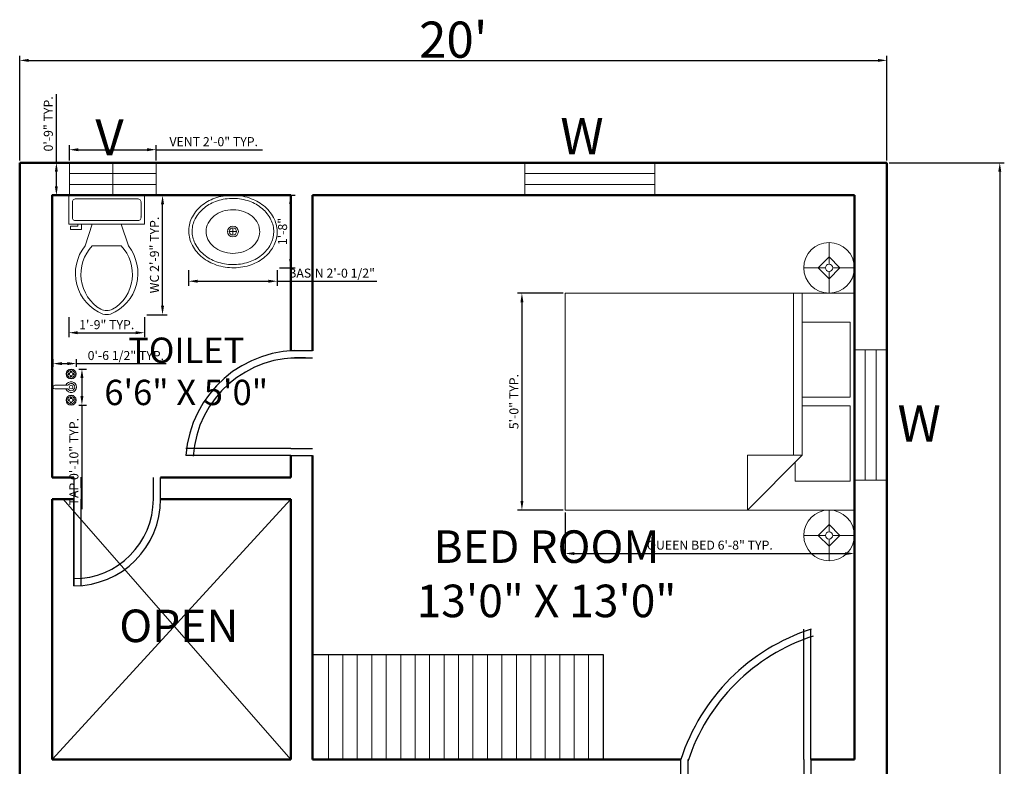
# Model space of a CAD drawing. Units: inches. Extents: x 995 to 2141, y 2161 to 2928.
# Tile 4 of 7: x 1051 to 1323, y 2711 to 2917. Entities that reach past the tile are written whole.
import ezdxf

# ---------------------------------------------------------------- set-up
doc = ezdxf.new("R2010")
doc.units = ezdxf.units.IN
for name, color, linetype, lineweight in [('A-ANNO-DIMS', 2, 'Continuous', 18), ('A-ANNO-TEXT', 7, 'Continuous', 18), ('A-AREA-IDEN', 7, 'Continuous', 25), ('A-DOOR', 3, 'Continuous', 25), ('A-FLOR-CASE', 8, 'Continuous', 25), ('A-FLOR-CASE-PATT', 252, 'Continuous', 13), ('A-FLOR-FIXT', 9, 'Continuous', 18), ('A-FLOR-OPEN', 8, 'Continuous', 13), ('A-FURN', 8, 'Continuous', 18), ('A-GLAZ', 4, 'Continuous', 18), ('A-WALL', 7, 'Continuous', 50)]:
    doc.layers.add(name, color=color, linetype=linetype, lineweight=lineweight)
doc.styles.get("Standard").update_dxf_attribs({"font": 'arial.ttf'})
doc.dimstyles.new('ISO-25', dxfattribs={"dimtxt": 2.5, "dimasz": 2.5, "dimexe": 1.25, "dimexo": 0.625, "dimtad": 1, "dimdec": 0, "dimlunit": 3, "dimtxsty": 'Standard', "dimcen": 2.5, "dimadec": 0, "dimazin": 0, "dimtfac": 1, "dimtdec": 0, "dimtmove": 0, "dimatfit": 3, "dimfxl": 1, "dimarcsym": 0})

# ---------------------------------------------------------------- blocks, each defined once
blk = doc.blocks.new('Sink - Oval top')
for p, q in [((-1, 0), (1, 0)), ((0, 1), (0, -1))]:
    blk.add_line(p, q)
for points in [[(-12.23, 0.39, 0.117634), (-11.46, -3.36, 0.104469), (-8.88, -6.8, 0.090016), (-5.08, -9.07, 0.08192), (-0.32, -10.02, 0.08192), (4.49, -9.38, 0.090016), (8.42, -7.36, 0.104469), (11.22, -4.09, 0.117634), (12.23, -0.39, 0.117634), (11.46, 3.36, 0.104469), (8.88, 6.8, 0.090016), (5.08, 9.07, 0.08192), (0.32, 10.02, 0.08192), (-4.49, 9.38, 0.090016), (-8.42, 7.36, 0.104469), (-11.22, 4.09, 0.117634)], [(-11.29, 0.16, 0.118622), (-10.52, -3.25, 0.104678), (-8.07, -6.36, 0.089562), (-4.54, -8.37, 0.081185), (-0.13, -9.15, 0.081185), (4.3, -8.49, 0.089562), (7.89, -6.58, 0.104678), (10.42, -3.55, 0.118622), (11.29, -0.16, 0.118622), (10.52, 3.25, 0.104678), (8.07, 6.36, 0.089562), (4.54, 8.37, 0.081185), (0.13, 9.15, 0.081185), (-4.3, 8.49, 0.089562), (-7.89, 6.58, 0.104678), (-10.42, 3.55, 0.118622)], [(-7.42, 0.08, 0.118283), (-6.91, -2.17, 0.104607), (-5.29, -4.21, 0.089718), (-2.97, -5.53, 0.081436), (-0.07, -6.04, 0.081436), (2.84, -5.59, 0.089718), (5.2, -4.33, 0.104607), (6.86, -2.32, 0.118283), (7.42, -0.08, 0.118283), (6.91, 2.17, 0.104607), (5.29, 4.21, 0.089718), (2.97, 5.53, 0.081436), (0.07, 6.04, 0.081436), (-2.84, 5.59, 0.089718), (-5.2, 4.33, 0.104607), (-6.86, 2.32, 0.118283)]]:
    blk.add_lwpolyline(points, format="xyb", close=True)
for radius in [1.5, 1]:
    blk.add_circle((0, 0), radius)
blk = doc.blocks.new('Toilet - top')
for p, q in [((9.5, -6), (9.5, -2)), ((-8, -8.5), (-8, -8)), ((-7, -8), (-7, -9.5)), ((-4, -8), (-6, -14)), ((4, -8), (6, -14)), ((-10, -8.5), (-8, -8.5)), ((-10, -9.5), (-10, -8.5)), ((-7, -9.5), (-10, -9.5)), ((4, -14), (-4, -14))]:
    blk.add_line(p, q)
blk.add_lwpolyline([(10.5, -8), (10.5, 0), (-10.5, 0), (-10.5, -8)], close=True)
for points in [[(-9.5, -2), (-9.5, -6)], [(8.5, -1), (-8.5, -1)], [(-8.5, -7), (8.5, -7)]]:
    blk.add_lwpolyline(points)
for centre, radius, start, end in [((-8.62, -1.88), 0.884, 81.8699, 188.1301), ((8.62, -1.88), 0.884, 351.8699, 98.1301), ((-8.62, -6.12), 0.884, 171.8699, 278.1301), ((8.62, -6.12), 0.884, 261.8699, 8.1301), ((3.52, -21.58), 12.17, 141.4691, 247.9714), ((4.2, -21.82), 11.33, 136.3677, 238.9468), ((-3.52, -21.58), 12.17, 292.0284, 38.5307), ((-4.2, -21.82), 11.33, 301.053, 43.6321), ((0, -27.88), 4, 245.7318, 294.2682), ((0, -29), 4, 254.8605, 285.1395)]:
    blk.add_arc(centre, radius, start, end)
blk = doc.blocks.new('Faucet - Bathroom top')
for p, q in [((-4.107, 0.125), (-4.375, 0.125)), ((-3.75, 0.4788), (-3.75, 0.75)), ((-3.5, 0.482), (-3.5, 0.75)), ((-3.1461, 0.125), (-2.875, 0.125)), ((3.143, 0.125), (2.875, 0.125)), ((3.5, 0.4788), (3.5, 0.75)), ((3.75, 0.482), (3.75, 0.75)), ((4.1039, 0.125), (4.375, 0.125)), ((-4.1039, -0.125), (-4.375, -0.125)), ((-3.75, -0.4821), (-3.75, -0.75)), ((-3.5, -0.4789), (-3.5, -0.75)), ((-3.143, -0.125), (-2.875, -0.125)), ((-0.5, -0.8639), (-0.5, -4.5)), ((0.5, -4.5), (0.5, -0.8631)), ((3.1461, -0.125), (2.875, -0.125)), ((3.5, -0.4821), (3.5, -0.75)), ((3.75, -0.4789), (3.75, -0.75)), ((4.107, -0.125), (4.375, -0.125))]:
    blk.add_line(p, q)
for centre, radius in [((-3.625, 0), 1.375), ((-4.625, 0), 0.2795), ((-3.625, 0), 0.5), ((-3.625, 1), 0.2795), ((-2.625, 0), 0.2795), ((0, 0), 0.5), ((3.625, 0), 1.375), ((2.625, 0), 0.2795), ((3.625, 0), 0.5), ((3.625, 1), 0.2795), ((4.625, 0), 0.2795), ((-3.625, -1), 0.2795), ((3.625, -1), 0.2795)]:
    blk.add_circle(centre, radius)
for centre, radius, start, end in [((-3.625, 0), 1, 105.2407, 164.2093), ((-3.625, 0), 1, 16.44125, 74.07887), ((0, 0), 1.5, 289.6514, 250.3603), ((0, 0), 1, 300.3431, 239.7554), ((3.625, 0), 1, 106.12, 164.0884), ((3.625, 0), 1, 16.23422, 73.90469), ((-3.625, 0), 1, 196.2342, 253.9047), ((-3.625, 0), 1, 286.12, 344.0884), ((3.625, 0), 1, 196.4413, 254.0789), ((3.625, 0), 1, 285.2407, 344.2093), ((0, -4.5), 0.5, 180, 0)]:
    blk.add_arc(centre, radius, start, end)
blk = doc.blocks.new('Bed - Queen')
for p, q in [((0, -80.00003), (0, 0)), ((0, 0), (59.99999, 0)), ((59.99999, 0), (59.99999, -80.00003)), ((7.99999, -1.2), (28.79998, -1.2)), ((7.99999, -14.4), (7.99999, -1.2)), ((28.79998, -1.2), (28.79998, -14.4)), ((31.19999, -1.2), (51.99999, -1.2)), ((31.19999, -14.4), (31.19999, -1.2)), ((51.99999, -1.2), (51.99999, -16.4)), ((0, -14.4), (44.8, -14.4)), ((59.99999, -29.6), (44.8, -14.4)), ((44.8, -14.4), (44.8, -29.6)), ((44.8, -16.8), (0, -16.8)), ((51.99999, -16.4), (46.79936, -16.4)), ((44.8, -29.6), (59.99999, -29.6)), ((59.99999, -80.00003), (0, -80.00003))]:
    blk.add_line(p, q)
blk = doc.blocks.new('Lamp - Table')
for p, q in [((0, 7), (0, 1)), ((0, 3), (-3, 0)), ((3, 0), (0, 3)), ((-1, 0), (-7, 0)), ((-3, 0), (0, -3)), ((0, -3), (3, 0)), ((1, 0), (7, 0)), ((0, -1), (0, -7))]:
    blk.add_line(p, q)
for radius in [7, 1]:
    blk.add_circle((0, 0), radius)
blk = doc.blocks.new('*D16')
at = {"layer": 'A-ANNO-DIMS', "color": 0, "lineweight": -2, "transparency": 16777216}
for p, q in [((1050.98, 2878.31), (1050.98, 2907.24)), ((1053.48, 2905.99), (1288.48, 2905.99)), ((1290.98, 2878.31), (1290.98, 2907.24))]:
    blk.add_line(p, q, dxfattribs=at)
at = {"layer": 'A-ANNO-DIMS', "color": 0, "transparency": 16777216}
for points in [[(1053.48, 2906.4), (1053.48, 2905.57), (1050.98, 2905.99)], [(1288.48, 2906.4), (1288.48, 2905.57), (1290.98, 2905.99)]]:
    blk.add_solid(points, dxfattribs=at)
at = {"layer": 'Defpoints', "color": 0, "transparency": 16777216}
for p in [(1290.98, 2905.99), (1050.98, 2877.69), (1290.98, 2877.69)]:
    blk.add_point(p, dxfattribs=at)
at = {"layer": 'A-ANNO-DIMS', "color": 0, "transparency": 16777216, "insert": (1170.98, 2911.72), "char_height": 2.5, "width": 4.2855, "attachment_point": 5}
blk.add_mtext("{\\H4x;20'}", dxfattribs=at)
blk = doc.blocks.new('*D17')
at = {"layer": 'A-ANNO-DIMS', "color": 0, "lineweight": -2, "transparency": 16777216}
for p, q in [((1291.61, 2877.69), (1323.48, 2877.69)), ((1322.23, 2875.19), (1322.23, 2280.19)), ((1291.61, 2277.69), (1323.48, 2277.69))]:
    blk.add_line(p, q, dxfattribs=at)
at = {"layer": 'A-ANNO-DIMS', "color": 0, "transparency": 16777216}
for points in [[(1321.81, 2875.19), (1322.65, 2875.19), (1322.23, 2877.69)], [(1321.81, 2280.19), (1322.65, 2280.19), (1322.23, 2277.69)]]:
    blk.add_solid(points, dxfattribs=at)
at = {"layer": 'Defpoints', "color": 0, "transparency": 16777216}
for p in [(1290.98, 2877.69), (1290.98, 2277.69), (1322.23, 2277.69)]:
    blk.add_point(p, dxfattribs=at)
at = {"layer": 'A-ANNO-DIMS', "color": 0, "transparency": 16777216, "insert": (1316.5, 2577.69), "char_height": 2.5, "attachment_point": 5, "rotation": 90}
blk.add_mtext("{\\H4x;50'}", dxfattribs=at)
blk = doc.blocks.new('WIN-36IN')
for p, q in [((0, 36), (0, 0)), ((9, 36), (0, 36)), ((3, 36), (3, 0)), ((6, 0), (6, 36)), ((9, 0), (9, 36)), ((0, 0), (9, 0))]:
    blk.add_line(p, q)
blk = doc.blocks.new('VENT-24IN')
for p, q in [((24, 9), (0, 9)), ((0, 9), (0, 0)), ((24, 9), (24, 0)), ((24, 6), (0, 6)), ((0, 3), (24, 3)), ((0, 0), (24, 0))]:
    blk.add_line(p, q)
blk = doc.blocks.new('*D32')
at = {"layer": 'A-ANNO-DIMS', "color": 0, "lineweight": -2, "transparency": 16777216}
for p, q in [((1064.74, 2878.31), (1064.74, 2882.54)), ((1067.24, 2881.29), (1086.24, 2881.29)), ((1088.74, 2878.31), (1088.74, 2882.54)), ((1088.74, 2881.29), (1118.14, 2881.29))]:
    blk.add_line(p, q, dxfattribs=at)
at = {"layer": 'A-ANNO-DIMS', "color": 0, "transparency": 16777216}
for points in [[(1067.24, 2881.71), (1067.24, 2880.87), (1064.74, 2881.29)], [(1086.24, 2881.71), (1086.24, 2880.87), (1088.74, 2881.29)]]:
    blk.add_solid(points, dxfattribs=at)
at = {"layer": 'Defpoints', "color": 0, "transparency": 16777216}
for p in [(1088.74, 2881.29), (1064.74, 2877.69), (1088.74, 2877.69)]:
    blk.add_point(p, dxfattribs=at)
at = {"layer": 'A-ANNO-DIMS', "color": 0, "transparency": 16777216, "insert": (1104.69, 2883.19), "char_height": 2.5, "attachment_point": 5}
blk.add_mtext('VENT 2\'-0" TYP.', dxfattribs=at)
blk = doc.blocks.new('*D33')
at = {"layer": 'A-ANNO-DIMS', "color": 0, "lineweight": -2, "transparency": 16777216}
for p, q in [((1061.14, 2877.69), (1061.14, 2896.68)), ((1064.11, 2877.69), (1059.89, 2877.69)), ((1061.14, 2871.19), (1061.14, 2875.19)), ((1064.11, 2868.69), (1059.89, 2868.69))]:
    blk.add_line(p, q, dxfattribs=at)
at = {"layer": 'A-ANNO-DIMS', "color": 0, "transparency": 16777216}
for points in [[(1060.72, 2875.19), (1061.55, 2875.19), (1061.14, 2877.69)], [(1060.72, 2871.19), (1061.55, 2871.19), (1061.14, 2868.69)]]:
    blk.add_solid(points, dxfattribs=at)
at = {"layer": 'Defpoints', "color": 0, "transparency": 16777216}
for p in [(1061.14, 2877.69), (1064.74, 2877.69), (1064.74, 2868.69)]:
    blk.add_point(p, dxfattribs=at)
at = {"layer": 'A-ANNO-DIMS', "color": 0, "transparency": 16777216, "insert": (1059.23, 2888.43), "char_height": 2.5, "attachment_point": 5, "rotation": 90}
blk.add_mtext('0\'-9" TYP.', dxfattribs=at)
blk = doc.blocks.new('*D42')
at = {"layer": 'A-ANNO-DIMS', "color": 0, "lineweight": -2, "transparency": 16777216}
for p, q in [((1086.19, 2868.69), (1091.77, 2868.69)), ((1090.52, 2838.14), (1090.52, 2866.19)), ((1086.19, 2835.64), (1091.77, 2835.64))]:
    blk.add_line(p, q, dxfattribs=at)
at = {"layer": 'A-ANNO-DIMS', "color": 0, "transparency": 16777216}
for points in [[(1090.1, 2866.19), (1090.94, 2866.19), (1090.52, 2868.69)], [(1090.1, 2838.14), (1090.94, 2838.14), (1090.52, 2835.64)]]:
    blk.add_solid(points, dxfattribs=at)
at = {"layer": 'Defpoints', "color": 0, "transparency": 16777216}
for p in [(1085.56, 2868.69), (1090.52, 2868.69), (1085.56, 2835.64)]:
    blk.add_point(p, dxfattribs=at)
at = {"layer": 'A-ANNO-DIMS', "color": 0, "transparency": 16777216, "insert": (1088.6, 2852.17), "char_height": 2.5, "attachment_point": 5, "rotation": 90}
blk.add_mtext('WC 2\'-9" TYP.', dxfattribs=at)
blk = doc.blocks.new('*D43')
at = {"layer": 'A-ANNO-DIMS', "color": 0, "lineweight": -2, "transparency": 16777216}
for p, q in [((1064.56, 2835.02), (1064.56, 2829.44)), ((1085.56, 2835.02), (1085.56, 2829.44)), ((1067.06, 2830.69), (1083.06, 2830.69))]:
    blk.add_line(p, q, dxfattribs=at)
at = {"layer": 'A-ANNO-DIMS', "color": 0, "transparency": 16777216}
for points in [[(1067.06, 2831.1), (1067.06, 2830.27), (1064.56, 2830.69)], [(1083.06, 2831.1), (1083.06, 2830.27), (1085.56, 2830.69)]]:
    blk.add_solid(points, dxfattribs=at)
at = {"layer": 'Defpoints', "color": 0, "transparency": 16777216}
for p in [(1064.56, 2835.64), (1085.56, 2835.64), (1085.56, 2830.69)]:
    blk.add_point(p, dxfattribs=at)
at = {"layer": 'A-ANNO-DIMS', "color": 0, "transparency": 16777216, "insert": (1075.06, 2832.59), "char_height": 2.5, "attachment_point": 5}
blk.add_mtext('1\'-9" TYP.', dxfattribs=at)
blk = doc.blocks.new('*D44')
at = {"layer": 'A-ANNO-DIMS', "color": 0, "lineweight": -2, "transparency": 16777216}
for p, q in [((1067.34, 2820.65), (1069.46, 2820.65)), ((1068.21, 2818.15), (1068.21, 2813.15)), ((1067.34, 2810.65), (1069.46, 2810.65)), ((1068.21, 2810.65), (1068.21, 2781.89))]:
    blk.add_line(p, q, dxfattribs=at)
at = {"layer": 'A-ANNO-DIMS', "color": 0, "transparency": 16777216}
for points in [[(1067.8, 2818.15), (1068.63, 2818.15), (1068.21, 2820.65)], [(1067.8, 2813.15), (1068.63, 2813.15), (1068.21, 2810.65)]]:
    blk.add_solid(points, dxfattribs=at)
at = {"layer": 'Defpoints', "color": 0, "transparency": 16777216}
for p in [(1066.71, 2820.65), (1066.71, 2810.65), (1068.21, 2810.65)]:
    blk.add_point(p, dxfattribs=at)
at = {"layer": 'A-ANNO-DIMS', "color": 0, "transparency": 16777216, "insert": (1066.31, 2795.02), "char_height": 2.5, "attachment_point": 5, "rotation": 90}
blk.add_mtext('TAP 0\'-10" TYP.', dxfattribs=at)
blk = doc.blocks.new('*D45')
at = {"layer": 'A-ANNO-DIMS', "color": 0, "lineweight": -2, "transparency": 16777216}
for p, q in [((1060.21, 2821.27), (1060.21, 2823.4)), ((1066.71, 2821.27), (1066.71, 2823.4)), ((1062.71, 2822.15), (1064.21, 2822.15)), ((1066.71, 2822.15), (1091.53, 2822.15))]:
    blk.add_line(p, q, dxfattribs=at)
at = {"layer": 'A-ANNO-DIMS', "color": 0, "transparency": 16777216}
for points in [[(1062.71, 2822.56), (1062.71, 2821.73), (1060.21, 2822.15)], [(1064.21, 2822.56), (1064.21, 2821.73), (1066.71, 2822.15)]]:
    blk.add_solid(points, dxfattribs=at)
at = {"layer": 'Defpoints', "color": 0, "transparency": 16777216}
for p in [(1060.21, 2820.65), (1066.71, 2822.15), (1066.71, 2820.65)]:
    blk.add_point(p, dxfattribs=at)
at = {"layer": 'A-ANNO-DIMS', "color": 0, "transparency": 16777216, "insert": (1080.37, 2824.06), "char_height": 2.5, "attachment_point": 5}
blk.add_mtext('0\'-6 1/2" TYP.', dxfattribs=at)
blk = doc.blocks.new('*D46')
at = {"layer": 'A-ANNO-DIMS', "color": 0, "lineweight": -2, "transparency": 16777216}
for p, q in [((1201.98, 2781), (1201.98, 2768.38)), ((1281.98, 2781), (1281.98, 2768.38)), ((1204.48, 2769.63), (1279.48, 2769.63))]:
    blk.add_line(p, q, dxfattribs=at)
at = {"layer": 'A-ANNO-DIMS', "color": 0, "transparency": 16777216}
for points in [[(1204.48, 2770.04), (1204.48, 2769.21), (1201.98, 2769.63)], [(1279.48, 2770.04), (1279.48, 2769.21), (1281.98, 2769.63)]]:
    blk.add_solid(points, dxfattribs=at)
at = {"layer": 'Defpoints', "color": 0, "transparency": 16777216}
for p in [(1201.98, 2781.63), (1281.98, 2781.63), (1281.98, 2769.63)]:
    blk.add_point(p, dxfattribs=at)
at = {"layer": 'A-ANNO-DIMS', "color": 0, "transparency": 16777216, "insert": (1241.98, 2771.62), "char_height": 2.5, "attachment_point": 5}
blk.add_mtext('QUEEN BED 6\'-8" TYP.', dxfattribs=at)
blk = doc.blocks.new('*D47')
at = {"layer": 'A-ANNO-DIMS', "color": 0, "lineweight": -2, "transparency": 16777216}
for p, q in [((1201.36, 2841.63), (1188.73, 2841.63)), ((1189.98, 2839.13), (1189.98, 2784.13)), ((1201.36, 2781.63), (1188.73, 2781.63))]:
    blk.add_line(p, q, dxfattribs=at)
at = {"layer": 'A-ANNO-DIMS', "color": 0, "transparency": 16777216}
for points in [[(1189.57, 2839.13), (1190.4, 2839.13), (1189.98, 2841.63)], [(1189.57, 2784.13), (1190.4, 2784.13), (1189.98, 2781.63)]]:
    blk.add_solid(points, dxfattribs=at)
at = {"layer": 'Defpoints', "color": 0, "transparency": 16777216}
for p in [(1201.98, 2841.63), (1189.98, 2781.63), (1201.98, 2781.63)]:
    blk.add_point(p, dxfattribs=at)
at = {"layer": 'A-ANNO-DIMS', "color": 0, "transparency": 16777216, "insert": (1188.08, 2811.63), "char_height": 2.5, "attachment_point": 5, "rotation": 90}
blk.add_mtext('5\'-0" TYP.', dxfattribs=at)
blk = doc.blocks.new('*D50')
at = {"layer": 'A-ANNO-DIMS', "color": 0, "lineweight": -2, "transparency": 16777216}
for p, q in [((1097.72, 2847.98), (1097.72, 2843.67)), ((1122.27, 2847.98), (1122.27, 2843.67)), ((1100.22, 2844.92), (1119.77, 2844.92)), ((1122.27, 2844.92), (1149.84, 2844.92))]:
    blk.add_line(p, q, dxfattribs=at)
at = {"layer": 'A-ANNO-DIMS', "color": 0, "transparency": 16777216}
for points in [[(1100.22, 2845.34), (1100.22, 2844.51), (1097.72, 2844.92)], [(1119.77, 2845.34), (1119.77, 2844.51), (1122.27, 2844.92)]]:
    blk.add_solid(points, dxfattribs=at)
at = {"layer": 'Defpoints', "color": 0, "transparency": 16777216}
for p in [(1097.72, 2848.6), (1122.27, 2848.6), (1122.27, 2844.92)]:
    blk.add_point(p, dxfattribs=at)
at = {"layer": 'A-ANNO-DIMS', "color": 0, "transparency": 16777216, "insert": (1137.31, 2846.84), "char_height": 2.5, "attachment_point": 5}
blk.add_mtext('BASIN 2\'-0 1/2"', dxfattribs=at)
blk = doc.blocks.new('*D51')
at = {"layer": 'A-ANNO-DIMS', "color": 0, "lineweight": -2, "transparency": 16777216}
for p, q in [((1122.9, 2868.74), (1127.21, 2868.74)), ((1125.96, 2851.1), (1125.96, 2866.24)), ((1122.9, 2848.6), (1127.21, 2848.6))]:
    blk.add_line(p, q, dxfattribs=at)
at = {"layer": 'A-ANNO-DIMS', "color": 0, "transparency": 16777216}
for points in [[(1125.54, 2866.24), (1126.37, 2866.24), (1125.96, 2868.74)], [(1125.54, 2851.1), (1126.37, 2851.1), (1125.96, 2848.6)]]:
    blk.add_solid(points, dxfattribs=at)
at = {"layer": 'Defpoints', "color": 0, "transparency": 16777216}
for p in [(1122.27, 2868.74), (1125.96, 2868.74), (1122.27, 2848.6)]:
    blk.add_point(p, dxfattribs=at)
at = {"layer": 'A-ANNO-DIMS', "color": 0, "transparency": 16777216, "insert": (1124.06, 2858.67), "char_height": 2.5, "attachment_point": 5, "rotation": 90}
blk.add_mtext('1\'-8"', dxfattribs=at)

msp = doc.modelspace()

# ---------------------------------------------------------------- hatches: boundary and pattern name
at = {"layer": 'A-FLOR-CASE-PATT'}
h = msp.add_hatch(dxfattribs=at)
h.set_pattern_fill('ANSI31', color=256, scale=1.260308, angle=45, style=0)
h.paths.add_polyline_path([(1134.43, 2712.69), (1210.43, 2712.69), (1210.43, 2741.69), (1134.43, 2741.69)])

# ---------------------------------------------------------------- linework, layer by layer
at = {"layer": 'A-DOOR'}
for p, q in [((1131.98, 2825.69), (1125.98, 2825.69)), ((1131.98, 2823.69), (1125.98, 2823.69)), ((1125.98, 2798.69), (1096.98, 2798.69)), ((1125.98, 2798.69), (1131.98, 2798.69)), ((1125.98, 2796.69), (1096.98, 2796.69)), ((1125.98, 2796.69), (1131.98, 2796.69)), ((1065.95, 2790.69), (1065.98, 2784.69)), ((1067.95, 2790.7), (1067.98, 2784.7)), ((1087.98, 2784.69), (1087.98, 2790.69)), ((1089.98, 2784.69), (1089.98, 2790.69)), ((1065.98, 2784.69), (1065.98, 2760.69)), ((1065.98, 2760.69), (1065.98, 2784.69)), ((1067.98, 2760.69), (1067.98, 2784.69)), ((1267.98, 2712.69), (1267.98, 2748.69)), ((1269.98, 2712.69), (1269.98, 2748.69)), ((1233.98, 2706.69), (1233.98, 2712.69)), ((1235.98, 2706.69), (1235.98, 2712.69)), ((1267.98, 2712.69), (1267.98, 2706.69)), ((1269.98, 2712.69), (1269.98, 2706.69))]:
    msp.add_line(p, q, dxfattribs=at)
for centre, radius, start, end in [((1128.08, 2794.6), 31.16, 86.1506, 176.1506), ((1128.08, 2794.6), 29.16, 86.1506, 176.1506), ((1065.98, 2784.69), 24, 270, 0), ((1065.98, 2784.69), 22, 270, 0), ((1287.19, 2695.49), 55.92, 107.9185, 162.0815), ((1287.19, 2695.49), 53.92, 107.9185, 162.0815)]:
    msp.add_arc(centre, radius, start, end, dxfattribs=at)
at = {"layer": 'A-FLOR-CASE'}
for p, q in [((1131.98, 2741.69), (1212.43, 2741.69)), ((1212.43, 2741.69), (1212.43, 2712.69))]:
    msp.add_line(p, q, dxfattribs=at)
at = {"layer": 'A-FLOR-OPEN'}
for p, q in [((1059.98, 2712.69), (1125.98, 2784.69)), ((1125.98, 2712.69), (1062.98, 2784.69))]:
    msp.add_line(p, q, dxfattribs=at)
at = {"layer": 'A-GLAZ'}
for p, q in [((1076.74, 2868.69), (1076.74, 2877.69)), ((1088.74, 2877.69), (1088.74, 2868.69))]:
    msp.add_line(p, q, dxfattribs=at)
at = {"layer": 'A-WALL'}
for p, q in [((1050.98, 2877.69), (1290.98, 2877.69)), ((1050.98, 2277.69), (1050.98, 2877.69)), ((1290.98, 2877.69), (1290.98, 2277.69)), ((1059.98, 2868.69), (1125.98, 2868.69)), ((1059.98, 2790.69), (1059.98, 2868.69)), ((1125.98, 2868.69), (1125.98, 2825.69)), ((1131.98, 2868.69), (1131.98, 2825.69)), ((1131.98, 2868.69), (1281.98, 2868.69)), ((1281.98, 2868.69), (1281.98, 2712.69)), ((1125.98, 2790.69), (1125.98, 2796.69)), ((1125.98, 2796.69), (1125.98, 2790.69)), ((1131.98, 2796.69), (1131.98, 2712.69)), ((1059.98, 2790.69), (1065.95, 2790.69)), ((1089.98, 2790.69), (1125.98, 2790.69)), ((1059.98, 2784.69), (1065.98, 2784.69)), ((1059.98, 2712.69), (1059.98, 2784.69)), ((1059.98, 2784.69), (1065.98, 2784.69)), ((1089.98, 2784.69), (1125.98, 2784.69)), ((1125.98, 2784.69), (1125.98, 2712.69)), ((1125.98, 2784.69), (1125.98, 2712.69)), ((1059.98, 2712.69), (1125.98, 2712.69)), ((1131.98, 2712.69), (1233.98, 2712.69)), ((1281.98, 2712.69), (1269.98, 2712.69)), ((1269.98, 2712.69), (1281.98, 2712.69))]:
    msp.add_line(p, q, dxfattribs=at)

# ---------------------------------------------------------------- block references
at = {"layer": 'A-FLOR-FIXT'}
for name, p in [('Toilet - top', (1075.06, 2868.69)), ('Sink - Oval top', (1110, 2858.67))]:
    msp.add_blockref(name, p, dxfattribs=at)
at = {"layer": 'A-FLOR-FIXT', "rotation": 270}
msp.add_blockref('Faucet - Bathroom top', (1065.21, 2815.65), dxfattribs=at)
at = {"layer": 'A-FURN', "rotation": 270}
for name, p in [('Lamp - Table', (1274.98, 2848.63)), ('Bed - Queen', (1281.98, 2841.63)), ('Lamp - Table', (1274.98, 2774.63))]:
    msp.add_blockref(name, p, dxfattribs=at)
at = {"layer": 'A-GLAZ'}
for name, p in [('VENT-24IN', (1064.74, 2868.69)), ('WIN-36IN', (1281.98, 2789.91))]:
    msp.add_blockref(name, p, dxfattribs=at)
at = {"layer": 'A-GLAZ', "rotation": 269.9999999999985}
msp.add_blockref('WIN-36IN', (1190.75, 2877.7), dxfattribs=at)

# ---------------------------------------------------------------- texts
at = {"layer": 'A-ANNO-TEXT', "char_height": 10, "attachment_point": 1}
for s, insert in [('V', (1071.92, 2889.71)), ('W', (1200.61, 2890.04)), ('W', (1293.93, 2810.6))]:
    msp.add_mtext_dynamic_manual_height_columns(s, width=112.484, gutter_width=12.5, heights=[0], dxfattribs=dict(at, insert=insert))
at = {"layer": 'A-AREA-IDEN', "attachment_point": 1}
for s, width, insert, char_height in [('\\pxqc;TOILET\\P6\'6" X 5\'0"', 53.0246, (1070.56, 2829.34), 7), ('\\pxqc;BED ROOM ^J13\'0" X 13\'0"', 109.7687, (1141.9, 2776.03), 9), ('\\pxqc;OPEN ', 52.2467, (1068.92, 2754.13), 9)]:
    msp.add_mtext_dynamic_manual_height_columns(s, width=width, gutter_width=12.5, heights=[0], dxfattribs=dict(at, insert=insert, char_height=char_height))

# ---------------------------------------------------------------- dimensions: what is measured, and where the dimension line sits
at = {"layer": 'A-ANNO-DIMS'}
for base, p1, p2, text, override, picture, middle in [((1290.98, 2905.99), (1050.98, 2877.69), (1290.98, 2877.69), "{\\H4x;20'}", {"dimclrd": 0, "dimclre": 0, "dimclrt": 0}, '*D16', (1170.98, 2911.72)), ((1088.74, 2881.29), (1064.74, 2877.69), (1088.74, 2877.69), 'VENT <> TYP.', {"dimdec": 1, "dimlfac": 1, "dimrnd": 0, "dimzin": 1, "dimdsep": 46, "dimlunit": 4, "dimfrac": 2}, '*D32', (1104.69, 2883.19)), ((1122.2749, 2844.9222), (1097.724, 2848.6048), (1122.2749, 2848.6048), 'BASIN <>', {"dimdec": 1, "dimlfac": 1, "dimrnd": 0, "dimzin": 1, "dimdsep": 46, "dimlunit": 4, "dimfrac": 2}, '*D50', (1137.3056, 2846.8398)), ((1085.56, 2830.69), (1064.56, 2835.64), (1085.56, 2835.64), '<> TYP.', {"dimdec": 1, "dimlfac": 1, "dimrnd": 0, "dimzin": 1, "dimdsep": 46, "dimlunit": 4, "dimfrac": 2}, '*D43', (1075.06, 2832.59)), ((1066.71, 2822.15), (1060.21, 2820.65), (1066.71, 2820.65), '<> TYP.', {"dimdec": 1, "dimlfac": 1, "dimrnd": 0, "dimzin": 1, "dimdsep": 46, "dimlunit": 4, "dimfrac": 2}, '*D45', (1080.37, 2824.06)), ((1281.98, 2769.63), (1201.98, 2781.63), (1281.98, 2781.63), 'QUEEN BED <> TYP.', {"dimdec": 1, "dimlfac": 1, "dimrnd": 0, "dimzin": 1, "dimdsep": 46, "dimlunit": 4, "dimfrac": 2}, '*D46', (1241.98, 2771.62))]:
    dim = msp.add_linear_dim(base=base, p1=p1, p2=p2, text=text, dimstyle='ISO-25', override=override, dxfattribs=at)
    dim.commit()
    dim.dimension.update_dxf_attribs({"geometry": picture, "text_midpoint": middle})
for base, p1, p2, angle, text, override, picture, middle in [((1061.14, 2877.69), (1064.74, 2868.69), (1064.74, 2877.69), 90, '<> TYP.', {"dimdec": 1, "dimlfac": 1, "dimrnd": 0, "dimzin": 1, "dimdsep": 46, "dimlunit": 4, "dimfrac": 2}, '*D33', (1059.23, 2888.43)), ((1322.23, 2277.69), (1290.98, 2877.69), (1290.98, 2277.69), 90, "{\\H4x;50'}", {"dimclrd": 0, "dimclre": 0, "dimclrt": 0}, '*D17', (1316.5, 2577.69)), ((1090.5188, 2868.689), (1085.5619, 2835.6427), (1085.5619, 2868.689), 90, 'WC <> TYP.', {"dimdec": 1, "dimlfac": 1, "dimrnd": 0, "dimzin": 1, "dimdsep": 46, "dimlunit": 4, "dimfrac": 2}, '*D42', (1088.6012, 2852.1658)), ((1189.98, 2781.63), (1201.98, 2841.63), (1201.98, 2781.63), 270, '<> TYP.', {"dimdec": 1, "dimlfac": 1, "dimrnd": 0, "dimzin": 1, "dimdsep": 46, "dimlunit": 4, "dimfrac": 2}, '*D47', (1188.08, 2811.63)), ((1068.21, 2810.65), (1066.71, 2820.65), (1066.71, 2810.65), 270, 'TAP <> TYP.', {"dimdec": 1, "dimlfac": 1, "dimrnd": 0, "dimzin": 1, "dimdsep": 46, "dimlunit": 4, "dimfrac": 2}, '*D44', (1066.31, 2795.02))]:
    dim = msp.add_linear_dim(base=base, p1=p1, p2=p2, angle=angle, text=text, dimstyle='ISO-25', override=override, dxfattribs=at)
    dim.commit()
    dim.dimension.update_dxf_attribs({"geometry": picture, "text_midpoint": middle})
dim = msp.add_linear_dim(base=(1125.96, 2868.74), p1=(1122.27, 2848.6), p2=(1122.27, 2868.74), angle=90, dimstyle='ISO-25', override={"dimdec": 1, "dimlfac": 1, "dimrnd": 0, "dimzin": 1, "dimdsep": 46, "dimlunit": 4, "dimfrac": 2}, dxfattribs=at)
dim.commit()
dim.dimension.update_dxf_attribs({"geometry": '*D51', "text_midpoint": (1124.06, 2858.67)})

doc.saveas('drawing.dxf')
